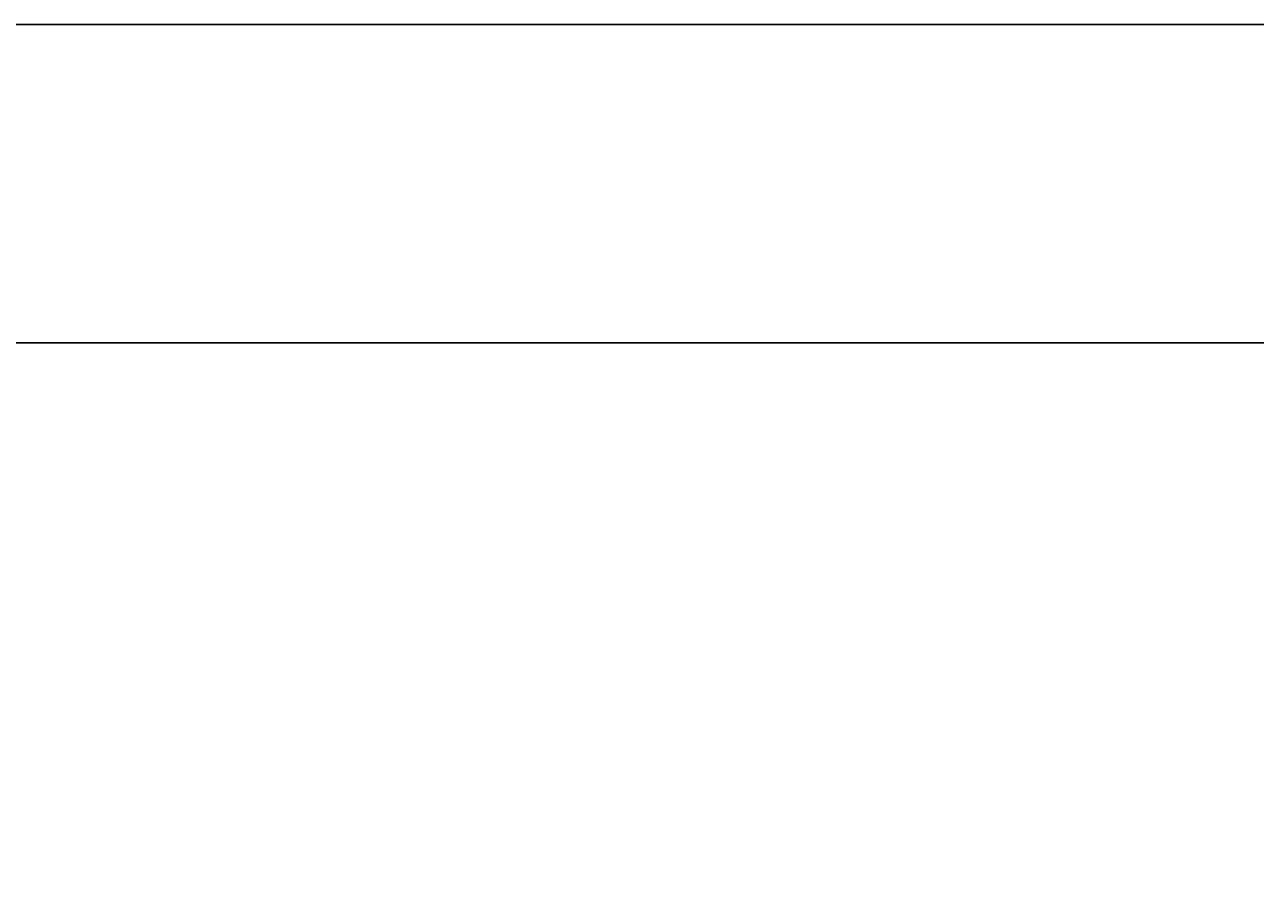
# Model space of a CAD drawing. Units: inches. Extents: x 1998 to 2588, y 1139 to 1977.
# Tile 49 of 134: x 2282 to 2313, y 1615 to 1637. Entities that reach past the tile are written whole.
import ezdxf

# ---------------------------------------------------------------- set-up
doc = ezdxf.new("R2010")
doc.units = ezdxf.units.IN
doc.layers.add('A-ANNO-DIMS', color=2, linetype='Continuous', lineweight=18)
doc.styles.get("Standard").update_dxf_attribs({"font": 'arial.ttf'})
doc.dimstyles.get("Standard").update_dxf_attribs({"dimtxt": 0.18, "dimasz": 0.18, "dimexe": 0.18, "dimexo": 0.0625, "dimgap": 0.09, "dimtad": 0, "dimtih": 1, "dimtoh": 1, "dimdec": 4, "dimzin": 0, "dimdsep": 46, "dimtxsty": 'Standard', "dimcen": 0.09, "dimadec": 0, "dimazin": 0, "dimtfac": 1, "dimtdec": 4, "dimtofl": 0, "dimtmove": 0, "dimatfit": 3, "dimfxl": 1, "dimtolj": 1, "dimtzin": 0, "dimarcsym": 0})

# ---------------------------------------------------------------- blocks, each defined once
blk = doc.blocks.new('*D30')
at = {"layer": 'A-ANNO-DIMS', "color": 0, "lineweight": -2, "transparency": 16777216}
for p, q in [((2407.91, 1636.732), (1997.843, 1636.732)), ((1998.023, 1636.552), (1998.023, 1615.913)), ((1998.023, 1594.912), (1998.023, 1615.552)), ((2407.91, 1594.732), (1997.843, 1594.732))]:
    blk.add_line(p, q, dxfattribs=at)
at = {"layer": 'A-ANNO-DIMS', "color": 0, "transparency": 16777216}
for points in [[(1997.993, 1636.552), (1998.053, 1636.552), (1998.023, 1636.732)], [(1997.993, 1594.912), (1998.053, 1594.912), (1998.023, 1594.732)]]:
    blk.add_solid(points, dxfattribs=at)
at = {"layer": 'Defpoints', "color": 0, "transparency": 16777216}
for p in [(1998.023, 1636.732), (2407.973, 1636.732), (2407.973, 1594.732)]:
    blk.add_point(p, dxfattribs=at)
at = {"layer": 'A-ANNO-DIMS', "color": 0, "transparency": 16777216, "insert": (1998.023, 1615.732), "char_height": 0.18, "attachment_point": 5}
blk.add_mtext('\\A1;42', dxfattribs=at)
blk = doc.blocks.new('*D39')
at = {"layer": 'A-ANNO-DIMS', "color": 0, "lineweight": -2, "transparency": 16777216}
for p, q in [((2115.035, 1628.742), (2588.309, 1628.742)), ((2588.129, 1628.562), (2588.129, 1612.685)), ((2588.129, 1596.444), (2588.129, 1612.321)), ((2115.035, 1596.264), (2588.309, 1596.264))]:
    blk.add_line(p, q, dxfattribs=at)
at = {"layer": 'A-ANNO-DIMS', "color": 0, "transparency": 16777216}
for points in [[(2588.099, 1628.562), (2588.159, 1628.562), (2588.129, 1628.742)], [(2588.099, 1596.444), (2588.159, 1596.444), (2588.129, 1596.264)]]:
    blk.add_solid(points, dxfattribs=at)
at = {"layer": 'Defpoints', "color": 0, "transparency": 16777216}
for p in [(2114.973, 1628.742), (2588.129, 1628.742), (2114.973, 1596.264)]:
    blk.add_point(p, dxfattribs=at)
at = {"layer": 'A-ANNO-DIMS', "color": 0, "transparency": 16777216, "insert": (2588.129, 1612.503), "char_height": 0.18, "attachment_point": 5}
blk.add_mtext('\\A1;32.48', dxfattribs=at)

msp = doc.modelspace()

# ---------------------------------------------------------------- dimensions: what is measured, and where the dimension line sits
at = {"layer": 'A-ANNO-DIMS'}
for base, p1, p2, override, picture, middle in [((1998.0229, 1636.7324), (2407.9729, 1594.7324), (2407.9729, 1636.7324), {"dimdec": 0, "dimlfac": 1, "dimrnd": 0, "dimzin": 0, "dimdsep": 46, "dimlunit": 2}, '*D30', (1998.0229, 1615.7324)), ((2588.1286, 1628.7416), (2114.9729, 1596.2642), (2114.9729, 1628.7416), {"dimdec": 2, "dimlfac": 1, "dimrnd": 0, "dimzin": 0, "dimdsep": 46, "dimlunit": 2}, '*D39', (2588.1286, 1612.5029))]:
    dim = msp.add_linear_dim(base=base, p1=p1, p2=p2, angle=90, dimstyle='Standard', override=override, dxfattribs=at)
    dim.commit()
    dim.dimension.update_dxf_attribs({"geometry": picture, "text_midpoint": middle})

doc.saveas('drawing.dxf')
